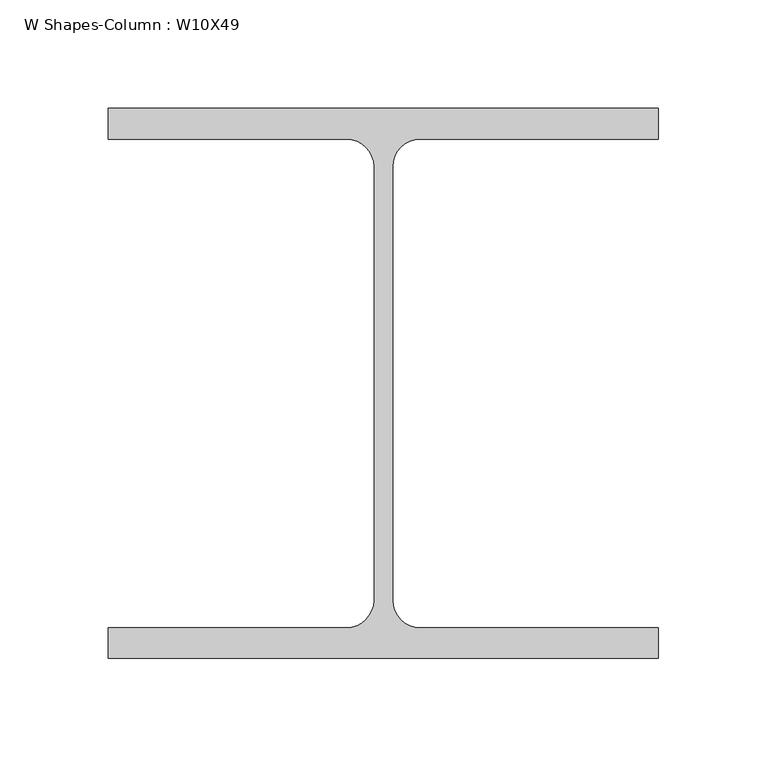
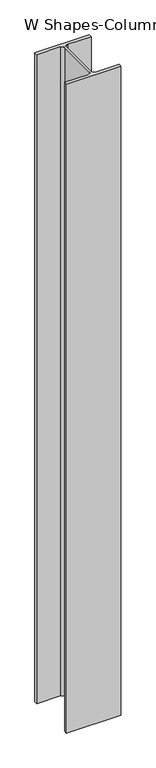
"""IFC4 building model written with IfcOpenShell, lengths in millimetres: column geometry, W Shapes-Column : W10X49."""

from ifc_helpers import new_model, si_unit, point, frame, frame_2d, origin, place, context, project, spatial, polyline, circle_curve, trimmed, segment, composite_curve, outline, extrude, source, transform, mapped, element, save


def w_shapes_column_w10x49_28d960f7(model_context):
    return source(origin(), model_context, "Body", "SweptSolid", [
        extrude(outline(composite_curve([segment(polyline([(127.0, 127.0), (127.0, 112.776), (17.018, 112.776)]), True, "CONTINUOUS"), segment(trimmed(circle_curve(frame_2d((17.018, 100.076)), 12.7), [point((17.018, 112.776))], [point((4.318, 100.076))], True, "CARTESIAN"), True, "CONTINUOUS"), segment(polyline([(4.318, 100.076), (4.318, -100.076)]), True, "CONTINUOUS"), segment(trimmed(circle_curve(frame_2d((17.018, -100.076)), 12.7), [point((4.318, -100.076))], [point((17.018, -112.776))], True, "CARTESIAN"), True, "CONTINUOUS"), segment(polyline([(17.018, -112.776), (127.0, -112.776), (127.0, -127.0), (-127.0, -127.0), (-127.0, -112.776), (-17.018, -112.776)]), True, "CONTINUOUS"), segment(trimmed(circle_curve(frame_2d((-17.018, -100.076)), 12.7), [point((-17.018, -112.776))], [point((-4.318, -100.076))], True, "CARTESIAN"), True, "CONTINUOUS"), segment(polyline([(-4.318, -100.076), (-4.318, 100.076)]), True, "CONTINUOUS"), segment(trimmed(circle_curve(frame_2d((-17.018, 100.076)), 12.7), [point((-4.318, 100.076))], [point((-17.018, 112.776))], True, "CARTESIAN"), True, "CONTINUOUS"), segment(polyline([(-17.018, 112.776), (-127.0, 112.776), (-127.0, 127.0), (127.0, 127.0)]), True, "CONTINUOUS")], self_intersect=False)), frame((0.0, 0.0, 6400.8), z_axis=(0.0, 0.0, 1.0), x_axis=(1.0, 0.0, 0.0)), (0.0, 0.0, 1.0), 3200.4),
    ])


if __name__ == "__main__":
    model = new_model("IFC4")
    model_context = context("Model", 3, world=origin())
    ifc_project = project(units=[si_unit("LENGTHUNIT", "METRE", prefix="MILLI")], contexts=[model_context])
    site = spatial("IfcSite", under=ifc_project)
    building = spatial("IfcBuilding", under=site)
    placement = place(None, origin())
    w_shapes_column_w10x49_shape = w_shapes_column_w10x49_28d960f7(model_context)
    element("IfcColumn", 1, ObjectType="W Shapes-Column : W10X49", at=placement, inside=building, context=model_context, shape_type="MappedRepresentation", body=[
        mapped(w_shapes_column_w10x49_shape, transform((0.0, 0.0, 0.0), x_axis=(1.0, 0.0, 0.0), y_axis=(0.0, 1.0, 0.0), z_axis=(0.0, 0.0, 1.0))),
    ])
    save(model, "model.ifc")

# Revit data of these elements
# Type "W Shapes-Column : W10X49"
#   Section Name Key = "W10x49"
#   Assembly Code = "B10"
#   Width = 10.000"
#   Web Thickness = 0.340"
#   Web Fillet = 0.500"
#   Warping Constant = 2070.00 in⁶
#   Torsional Moment of Inertia = 1.39 in⁴
#   Section Area = 14.40 in²
#   Plastic Modulus weak axis = 28.30 in³
#   Plastic Modulus strong axis = 60.40 in³
#   Perimeter = 58.50 ft²/ft
#   Nominal Weight = 49.00 lbf/ft
#   Moment of Inertia weak axis = 93.40 in⁴
#   Moment of Inertia strong axis = 272.00 in⁴
#   Height = 10.000"
#   Flange Thickness = 0.560"
#   Elastic Modulus weak axis = 18.70 in³
#   Elastic Modulus strong axis = 54.60 in³
#   Centroid Vertical = 5.000"
#   Centroid Horizontal = 5.000"
#   Structural Material [instance default] = Steel ASTM A992
#   Principal Axes Angle = 0
# Element 1 (IfcColumn, "W Shapes-Column : W10X49")
#   Materials on its faces: "Steel ASTM A992"
# Materials
#   "Steel ASTM A992": class "Metal", colour RGB 199 199 199, transparency 0, Description = "Structural steel 50ksi", Cost = 0
